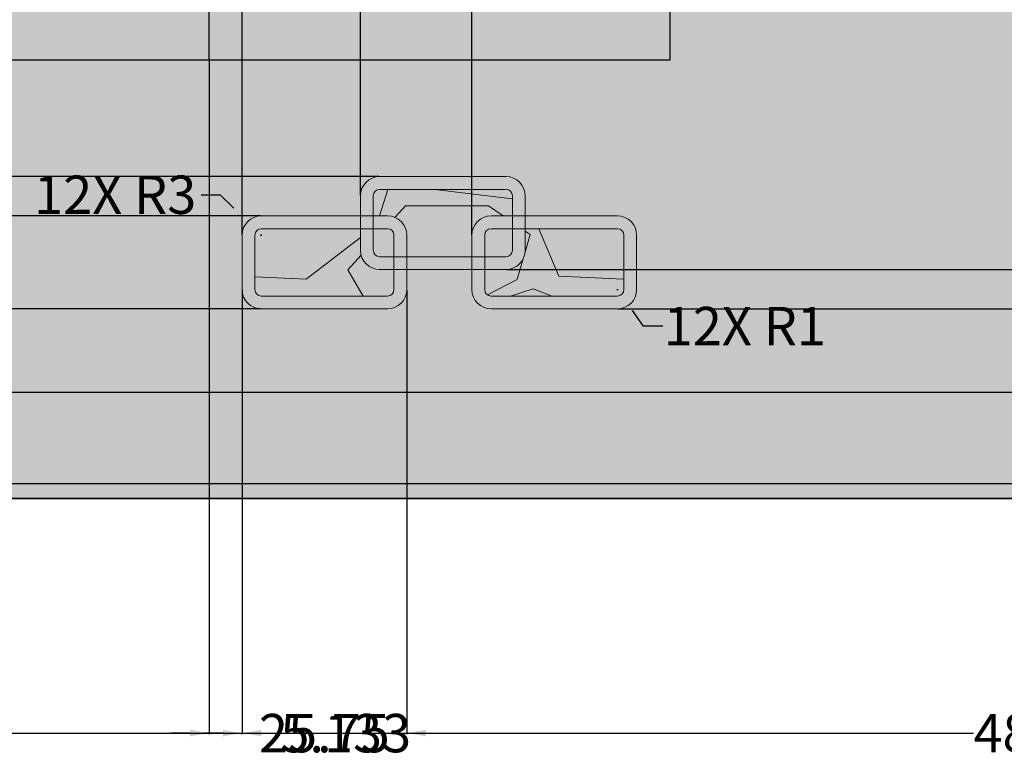
# Model space of a CAD drawing. Units: inches. Extents: x 126 to 726, y 86 to 888.
# Tile 2 of 13: x 270 to 424, y 86 to 202. Entities that reach past the tile are written whole.
import ezdxf

# ---------------------------------------------------------------- set-up
doc = ezdxf.new("R2010")
doc.units = ezdxf.units.IN
doc.header["$MEASUREMENT"] = 0
for name, color, linetype, lineweight in [('A-ANNO-DIMS', 2, 'Continuous', 18), ('A-ELEV', 7, 'Continuous', 35), ('A-ELEV-DECO', 7, 'Continuous', 18), ('A-ELEV-PATT', 8, 'Continuous', 13), ('A-GLAZ', 4, 'Continuous', 25)]:
    doc.layers.add(name, color=color, linetype=linetype, lineweight=lineweight)
doc.styles.get("Standard").update_dxf_attribs({"font": 'arial.ttf'})
doc.dimstyles.get("Standard").update_dxf_attribs({"dimtxt": 6, "dimasz": 3, "dimexe": 0.18, "dimexo": 0.0625, "dimgap": 0.09, "dimtad": 0, "dimtih": 1, "dimtoh": 1, "dimdec": 0, "dimzin": 0, "dimdsep": 46, "dimlunit": 3, "dimtxsty": 'Standard', "dimcen": 0.09, "dimadec": 0, "dimazin": 0, "dimtfac": 1, "dimtdec": 0, "dimtofl": 0, "dimtmove": 0, "dimatfit": 3, "dimfxl": 1, "dimtolj": 1, "dimtzin": 0, "dimarcsym": 0})

# ---------------------------------------------------------------- blocks, each defined once
blk = doc.blocks.new('WIN-FRAME')
for points in [[(72, 0), (0, 0), (0, 108), (72, 108)], [(63, 9), (9, 9), (9, 99), (63, 99)]]:
    blk.add_lwpolyline(points, close=True)
blk = doc.blocks.new('*D13')
at = {"layer": 'A-ANNO-DIMS', "color": 0, "lineweight": -2, "transparency": 16777216}
for p, q in [((665.97, 642.98), (665.97, 90.21)), ((185.97, 126.98), (185.97, 90.21)), ((188.97, 90.39), (419.15, 90.39)), ((662.97, 90.39), (432.8, 90.39))]:
    blk.add_line(p, q, dxfattribs=at)
at = {"layer": 'A-ANNO-DIMS', "color": 0, "transparency": 16777216}
for points in [[(188.97, 90.89), (188.97, 89.89), (185.97, 90.39)], [(662.97, 90.89), (662.97, 89.89), (665.97, 90.39)]]:
    blk.add_solid(points, dxfattribs=at)
at = {"layer": 'Defpoints', "color": 0, "transparency": 16777216}
for p in [(665.97, 643.04), (185.97, 127.04), (665.97, 90.39)]:
    blk.add_point(p, dxfattribs=at)
at = {"layer": 'A-ANNO-DIMS', "color": 0, "transparency": 16777216, "insert": (425.97, 90.39), "char_height": 6, "attachment_point": 5}
blk.add_mtext('\\A1;480', dxfattribs=at)
blk = doc.blocks.new('*D15')
at = {"layer": 'A-ANNO-DIMS', "color": 0, "lineweight": -2, "transparency": 16777216}
for p, q in [((299.6, 195.59), (149.14, 195.59)), ((149.32, 192.59), (149.32, 164.47)), ((149.32, 130.04), (149.32, 158.16)), ((185.91, 127.04), (149.14, 127.04))]:
    blk.add_line(p, q, dxfattribs=at)
at = {"layer": 'A-ANNO-DIMS', "color": 0, "transparency": 16777216}
for points in [[(148.82, 192.59), (149.82, 192.59), (149.32, 195.59)], [(148.82, 130.04), (149.82, 130.04), (149.32, 127.04)]]:
    blk.add_solid(points, dxfattribs=at)
at = {"layer": 'Defpoints', "color": 0, "transparency": 16777216}
for p in [(149.32, 195.59), (299.67, 195.59), (185.97, 127.04)]:
    blk.add_point(p, dxfattribs=at)
at = {"layer": 'A-ANNO-DIMS', "color": 0, "transparency": 16777216, "insert": (149.32, 161.31), "char_height": 6, "attachment_point": 5}
blk.add_mtext('\\A1;68.55', dxfattribs=at)
blk = doc.blocks.new('*D16')
at = {"layer": 'A-ANNO-DIMS', "color": 0, "lineweight": -2, "transparency": 16777216}
for p, q in [((299.6, 425.68), (149.14, 425.68)), ((149.32, 422.68), (149.32, 313.79)), ((149.32, 198.59), (149.32, 307.48)), ((299.6, 195.59), (149.14, 195.59))]:
    blk.add_line(p, q, dxfattribs=at)
at = {"layer": 'A-ANNO-DIMS', "color": 0, "transparency": 16777216}
for points in [[(148.82, 422.68), (149.82, 422.68), (149.32, 425.68)], [(148.82, 198.59), (149.82, 198.59), (149.32, 195.59)]]:
    blk.add_solid(points, dxfattribs=at)
at = {"layer": 'Defpoints', "color": 0, "transparency": 16777216}
for p in [(149.32, 425.68), (299.67, 425.68), (299.67, 195.59)]:
    blk.add_point(p, dxfattribs=at)
at = {"layer": 'A-ANNO-DIMS', "color": 0, "transparency": 16777216, "insert": (149.32, 310.64), "char_height": 6, "attachment_point": 5}
blk.add_mtext('\\A1;230.1', dxfattribs=at)
blk = doc.blocks.new('*D18')
at = {"layer": 'A-ANNO-DIMS', "color": 0, "lineweight": -2, "transparency": 16777216}
for p, q in [((431.28, 395.58), (149.14, 395.58)), ((149.32, 392.58), (149.32, 264.47)), ((149.32, 130.04), (149.32, 258.16)), ((185.91, 127.04), (149.14, 127.04))]:
    blk.add_line(p, q, dxfattribs=at)
at = {"layer": 'A-ANNO-DIMS', "color": 0, "transparency": 16777216}
for points in [[(148.82, 392.58), (149.82, 392.58), (149.32, 395.58)], [(148.82, 130.04), (149.82, 130.04), (149.32, 127.04)]]:
    blk.add_solid(points, dxfattribs=at)
at = {"layer": 'Defpoints', "color": 0, "transparency": 16777216}
for p in [(149.32, 395.58), (431.34, 395.58), (185.97, 127.04)]:
    blk.add_point(p, dxfattribs=at)
at = {"layer": 'A-ANNO-DIMS', "color": 0, "transparency": 16777216, "insert": (149.32, 261.31), "char_height": 6, "attachment_point": 5}
blk.add_mtext('\\A1;268.54', dxfattribs=at)
blk = doc.blocks.new('*D30')
at = {"layer": 'A-ANNO-DIMS', "color": 0, "lineweight": -2, "transparency": 16777216}
for p, q in [((299.6, 195.59), (149.14, 195.59)), ((149.32, 192.59), (149.32, 189.64)), ((149.32, 180.39), (149.32, 183.33)), ((326.24, 177.39), (149.14, 177.39))]:
    blk.add_line(p, q, dxfattribs=at)
at = {"layer": 'A-ANNO-DIMS', "color": 0, "transparency": 16777216}
for points in [[(148.82, 192.59), (149.82, 192.59), (149.32, 195.59)], [(148.82, 180.39), (149.82, 180.39), (149.32, 177.39)]]:
    blk.add_solid(points, dxfattribs=at)
at = {"layer": 'Defpoints', "color": 0, "transparency": 16777216}
for p in [(149.32, 195.59), (299.67, 195.59), (326.3, 177.39)]:
    blk.add_point(p, dxfattribs=at)
at = {"layer": 'A-ANNO-DIMS', "color": 0, "transparency": 16777216, "insert": (149.32, 186.49), "char_height": 6, "attachment_point": 5}
blk.add_mtext('\\A1;18.2', dxfattribs=at)
blk = doc.blocks.new('*D31')
at = {"layer": 'A-ANNO-DIMS', "color": 0, "lineweight": -2, "transparency": 16777216}
for p, q in [((299.67, 195.52), (299.67, 90.21)), ((304.8, 159.65), (304.8, 90.21)), ((296.67, 90.39), (293.67, 90.39)), ((307.8, 90.39), (310.8, 90.39))]:
    blk.add_line(p, q, dxfattribs=at)
at = {"layer": 'A-ANNO-DIMS', "color": 0, "transparency": 16777216}
for points in [[(296.67, 90.89), (296.67, 89.89), (299.67, 90.39)], [(307.8, 90.89), (307.8, 89.89), (304.8, 90.39)]]:
    blk.add_solid(points, dxfattribs=at)
at = {"layer": 'Defpoints', "color": 0, "transparency": 16777216}
for p in [(299.67, 195.59), (304.8, 159.71), (304.8, 90.39)]:
    blk.add_point(p, dxfattribs=at)
at = {"layer": 'A-ANNO-DIMS', "color": 0, "transparency": 16777216, "insert": (321.01, 90.39), "char_height": 6, "attachment_point": 5}
blk.add_mtext('\\A1;5.133', dxfattribs=at)
blk = doc.blocks.new('*D36')
at = {"layer": 'A-ANNO-DIMS', "color": 0, "lineweight": -2, "transparency": 16777216}
for p, q in [((304.8, 159.65), (304.8, 90.21)), ((330.55, 159.65), (330.55, 90.21)), ((301.8, 90.39), (298.8, 90.39)), ((333.55, 90.39), (336.55, 90.39))]:
    blk.add_line(p, q, dxfattribs=at)
at = {"layer": 'A-ANNO-DIMS', "color": 0, "transparency": 16777216}
for points in [[(301.8, 90.89), (301.8, 89.89), (304.8, 90.39)], [(333.55, 90.89), (333.55, 89.89), (330.55, 90.39)]]:
    blk.add_solid(points, dxfattribs=at)
at = {"layer": 'Defpoints', "color": 0, "transparency": 16777216}
for p in [(304.8, 159.71), (330.55, 159.71), (330.55, 90.39)]:
    blk.add_point(p, dxfattribs=at)
at = {"layer": 'A-ANNO-DIMS', "color": 0, "transparency": 16777216, "insert": (317.67, 90.39), "char_height": 6, "attachment_point": 5}
blk.add_mtext('\\A1;25.75', dxfattribs=at)
blk = doc.blocks.new('*D37')
at = {"layer": 'A-ANNO-DIMS', "color": 0, "lineweight": -2, "transparency": 16777216}
for p, q in [((307.74, 171.24), (149.14, 171.24)), ((149.32, 168.24), (149.32, 167.13)), ((149.32, 159.71), (149.32, 160.82)), ((307.74, 156.71), (149.14, 156.71))]:
    blk.add_line(p, q, dxfattribs=at)
at = {"layer": 'A-ANNO-DIMS', "color": 0, "transparency": 16777216}
for points in [[(148.82, 168.24), (149.82, 168.24), (149.32, 171.24)], [(148.82, 159.71), (149.82, 159.71), (149.32, 156.71)]]:
    blk.add_solid(points, dxfattribs=at)
at = {"layer": 'Defpoints', "color": 0, "transparency": 16777216}
for p in [(149.32, 171.24), (307.8, 171.24), (307.8, 156.71)]:
    blk.add_point(p, dxfattribs=at)
at = {"layer": 'A-ANNO-DIMS', "color": 0, "transparency": 16777216, "insert": (149.32, 163.98), "char_height": 6, "attachment_point": 5}
blk.add_mtext('\\A1;14.524', dxfattribs=at)
blk = doc.blocks.new('*D38')
at = {"layer": 'A-ANNO-DIMS', "color": 0, "lineweight": -2, "transparency": 16777216}
for p, q in [((304.8, 168.3), (304.8, 883.87)), ((307.8, 883.69), (320.3, 883.69)), ((323.3, 174.45), (323.3, 883.87)), ((323.3, 883.69), (326.3, 883.69))]:
    blk.add_line(p, q, dxfattribs=at)
at = {"layer": 'A-ANNO-DIMS', "color": 0, "transparency": 16777216}
for points in [[(307.8, 884.19), (307.8, 883.19), (304.8, 883.69)], [(320.3, 884.19), (320.3, 883.19), (323.3, 883.69)]]:
    blk.add_solid(points, dxfattribs=at)
at = {"layer": 'Defpoints', "color": 0, "transparency": 16777216}
for p in [(323.3, 883.69), (323.3, 174.39), (304.8, 168.24)]:
    blk.add_point(p, dxfattribs=at)
at = {"layer": 'A-ANNO-DIMS', "color": 0, "transparency": 16777216, "insert": (338.59, 883.69), "char_height": 6, "attachment_point": 5}
blk.add_mtext('\\A1;18.505', dxfattribs=at)
blk = doc.blocks.new('*D39')
at = {"layer": 'A-ANNO-DIMS', "color": 0, "lineweight": -2, "transparency": 16777216}
for p, q in [((323.3, 174.45), (323.3, 883.87)), ((326.3, 883.69), (337.74, 883.69)), ((340.74, 168.3), (340.74, 883.87)), ((340.74, 883.69), (343.74, 883.69))]:
    blk.add_line(p, q, dxfattribs=at)
at = {"layer": 'A-ANNO-DIMS', "color": 0, "transparency": 16777216}
for points in [[(326.3, 884.19), (326.3, 883.19), (323.3, 883.69)], [(337.74, 884.19), (337.74, 883.19), (340.74, 883.69)]]:
    blk.add_solid(points, dxfattribs=at)
at = {"layer": 'Defpoints', "color": 0, "transparency": 16777216}
for p in [(340.74, 883.69), (323.3, 174.39), (340.74, 168.24)]:
    blk.add_point(p, dxfattribs=at)
at = {"layer": 'A-ANNO-DIMS', "color": 0, "transparency": 16777216, "insert": (355.99, 883.69), "char_height": 6, "attachment_point": 5}
blk.add_mtext('\\A1;17.434', dxfattribs=at)
blk = doc.blocks.new('*D40')
at = {"layer": 'A-ANNO-DIMS', "color": 0, "lineweight": -2, "transparency": 16777216}
for p, q in [((702.62, 165.86), (702.62, 168.86)), ((702.62, 168.86), (705.62, 168.86)), ((346.12, 162.86), (702.8, 162.86)), ((363.55, 156.71), (702.8, 156.71)), ((702.62, 153.71), (702.62, 150.71))]:
    blk.add_line(p, q, dxfattribs=at)
at = {"layer": 'A-ANNO-DIMS', "color": 0, "transparency": 16777216}
for points in [[(702.12, 165.86), (703.12, 165.86), (702.62, 162.86)], [(702.12, 153.71), (703.12, 153.71), (702.62, 156.71)]]:
    blk.add_solid(points, dxfattribs=at)
at = {"layer": 'Defpoints', "color": 0, "transparency": 16777216}
for p in [(346.06, 162.86), (702.62, 162.86), (363.49, 156.71)]:
    blk.add_point(p, dxfattribs=at)
at = {"layer": 'A-ANNO-DIMS', "color": 0, "transparency": 16777216, "insert": (715.86, 168.86), "char_height": 6, "attachment_point": 5}
blk.add_mtext('\\A1;6.149', dxfattribs=at)
blk = doc.blocks.new('*D79')
at = {"layer": 'A-ANNO-DIMS', "color": 0, "lineweight": -2, "transparency": 16777216}
for p, q in [((149.32, 132.35), (149.32, 135.35)), ((437.91, 129.35), (149.14, 129.35)), ((485.91, 127.04), (149.14, 127.04)), ((149.32, 124.04), (149.32, 121.04)), ((149.32, 121.04), (146.32, 121.04))]:
    blk.add_line(p, q, dxfattribs=at)
at = {"layer": 'A-ANNO-DIMS', "color": 0, "transparency": 16777216}
for points in [[(148.82, 132.35), (149.82, 132.35), (149.32, 129.35)], [(148.82, 124.04), (149.82, 124.04), (149.32, 127.04)]]:
    blk.add_solid(points, dxfattribs=at)
at = {"layer": 'Defpoints', "color": 0, "transparency": 16777216}
for p in [(437.97, 129.35), (149.32, 127.04), (485.97, 127.04)]:
    blk.add_point(p, dxfattribs=at)
at = {"layer": 'A-ANNO-DIMS', "color": 0, "transparency": 16777216, "insert": (136.64, 121.04), "char_height": 6, "attachment_point": 5}
blk.add_mtext('\\A1;2.311', dxfattribs=at)
blk = doc.blocks.new('*D80')
at = {"layer": 'A-ANNO-DIMS', "color": 0, "lineweight": -2, "transparency": 16777216}
for p, q in [((437.91, 143.66), (149.14, 143.66)), ((149.32, 140.66), (149.32, 139.66)), ((149.32, 132.35), (149.32, 133.35)), ((437.91, 129.35), (149.14, 129.35))]:
    blk.add_line(p, q, dxfattribs=at)
at = {"layer": 'A-ANNO-DIMS', "color": 0, "transparency": 16777216}
for points in [[(148.82, 140.66), (149.82, 140.66), (149.32, 143.66)], [(148.82, 132.35), (149.82, 132.35), (149.32, 129.35)]]:
    blk.add_solid(points, dxfattribs=at)
at = {"layer": 'Defpoints', "color": 0, "transparency": 16777216}
for p in [(149.32, 143.66), (437.97, 143.66), (437.97, 129.35)]:
    blk.add_point(p, dxfattribs=at)
at = {"layer": 'A-ANNO-DIMS', "color": 0, "transparency": 16777216, "insert": (149.32, 136.51), "char_height": 6, "attachment_point": 5}
blk.add_mtext('\\A1;14.31', dxfattribs=at)
blk = doc.blocks.new('*D83')
at = {"layer": 'A-ANNO-DIMS', "color": 0, "lineweight": -2, "transparency": 16777216}
for p, q in [((298.38, 174.55), (301.38, 174.55)), ((301.38, 174.55), (303.52, 172.44)), ((307.71, 168.24), (307.89, 168.24)), ((307.8, 168.15), (307.8, 168.33))]:
    blk.add_line(p, q, dxfattribs=at)
at = {"layer": 'A-ANNO-DIMS', "color": 0, "transparency": 16777216}
blk.add_solid([(303.87, 172.8), (303.17, 172.09), (305.66, 170.34)], dxfattribs=at)
at = {"layer": 'Defpoints', "color": 0, "transparency": 16777216}
for p in [(305.66, 170.34), (307.8, 168.24)]:
    blk.add_point(p, dxfattribs=at)
at = {"layer": 'A-ANNO-DIMS', "color": 0, "transparency": 16777216, "insert": (284.96, 174.55), "char_height": 6, "attachment_point": 5}
blk.add_mtext('\\A1;12X R3', dxfattribs=at)
blk = doc.blocks.new('*D84')
at = {"layer": 'A-ANNO-DIMS', "color": 0, "lineweight": -2, "transparency": 16777216}
for p, q in [((363.4, 159.71), (363.58, 159.71)), ((363.49, 159.62), (363.49, 159.8)), ((367.57, 154.02), (365.82, 156.46)), ((370.57, 154.02), (367.57, 154.02))]:
    blk.add_line(p, q, dxfattribs=at)
at = {"layer": 'A-ANNO-DIMS', "color": 0, "transparency": 16777216}
blk.add_solid([(366.22, 156.75), (365.41, 156.17), (364.07, 158.9)], dxfattribs=at)
at = {"layer": 'Defpoints', "color": 0, "transparency": 16777216}
for p in [(363.49, 159.71), (364.07, 158.9)]:
    blk.add_point(p, dxfattribs=at)
at = {"layer": 'A-ANNO-DIMS', "color": 0, "transparency": 16777216, "insert": (383.41, 154.02), "char_height": 6, "attachment_point": 5}
blk.add_mtext('\\A1;12X R1', dxfattribs=at)

msp = doc.modelspace()

# ---------------------------------------------------------------- hatches: boundary and pattern name
at = {"layer": 'A-ELEV-PATT'}
h = msp.add_hatch(color=256, dxfattribs=at)
h.dxf.hatch_style = 1
h.paths.add_polyline_path([(437.9749, 499.1312), (485.9749, 499.1312), (485.9749, 501.4423), (437.9749, 501.4423), (437.9749, 513.4423), (485.9749, 513.4423), (485.9749, 515.7534), (437.9749, 515.7534), (437.9749, 527.7534), (485.9749, 527.7534), (485.9749, 530.0646), (437.9749, 530.0646), (437.9749, 542.0646), (485.9749, 542.0646), (485.9749, 544.3757), (437.9749, 544.3757), (437.9749, 556.3757), (485.9749, 556.3757), (485.9749, 558.6868), (437.9749, 558.6868), (437.9749, 570.6868), (485.9749, 570.6868), (485.9749, 572.9979), (437.9749, 572.9979), (437.9749, 584.9979), (485.9749, 584.9979), (485.9749, 587.309), (437.9749, 587.309), (437.9749, 595.0424), (429.9749, 595.0424), (429.9749, 607.0424), (437.9749, 607.0424), (437.9749, 615.9312), (437.9749, 630.2423), (437.9749, 642.2423), (485.9749, 642.2423), (485.9749, 644.5534), (437.9749, 644.5534), (437.9749, 656.5534), (485.9749, 656.5534), (485.9749, 658.8645), (437.9749, 658.8645), (437.9749, 670.8645), (485.9749, 670.8645), (485.9749, 673.1757), (437.9749, 673.1757), (437.9749, 685.1757), (485.9749, 685.1757), (485.9749, 687.4868), (437.9749, 687.4868), (437.9749, 699.4868), (485.9749, 699.4868), (485.9749, 701.7979), (437.9749, 701.7979), (437.9749, 713.7979), (485.9749, 713.7979), (485.9749, 716.109), (437.9749, 716.109), (437.9749, 728.109), (485.9749, 728.109), (485.9749, 730.4201), (437.9749, 730.4201), (437.9749, 742.4201), (485.9749, 742.4201), (485.9749, 744.7312), (437.9749, 744.7312), (437.9749, 756.7312), (485.9749, 756.7312), (485.9749, 759.0423), (437.9749, 759.0423), (437.9749, 771.0423), (485.9749, 771.0423), (485.9749, 773.3534), (437.9749, 773.3534), (437.9749, 785.3534), (485.9749, 785.3534), (485.9749, 787.6645), (437.9749, 787.6645), (437.9749, 799.6645), (485.9749, 799.6645), (485.9749, 801.9756), (437.9749, 801.9756), (437.9749, 811.2868), (485.9749, 811.2868), (485.9749, 813.9756), (437.9749, 813.9756), (437.9749, 825.9756), (485.9749, 825.9756), (485.9749, 835.0424), (233.9749, 835.0424), (233.9749, 606.5846), (185.9749, 606.5846), (185.9749, 597.5846), (233.9749, 597.5846), (233.9749, 585.5846), (185.9749, 585.5846), (185.9749, 580.5846), (233.9749, 580.5846), (233.9749, 568.5846), (185.9749, 568.5846), (185.9749, 563.5846), (431.3386, 563.5846), (431.3386, 545.5846), (233.9749, 545.5846), (233.9749, 413.5846), (431.3386, 413.5846), (431.3386, 395.5846), (185.9749, 395.5846), (185.9749, 386.5846), (233.9749, 386.5846), (233.9749, 374.5846), (185.9749, 374.5846), (185.9749, 369.5846), (233.9749, 369.5846), (233.9749, 357.5846), (185.9749, 357.5846), (185.9749, 352.5846), (233.9749, 352.5846), (233.9749, 340.5846), (185.9749, 340.5846), (185.9749, 331.5846), (233.9749, 331.5846), (233.9749, 127.0424), (485.9749, 127.0424), (485.9749, 129.3535), (437.9749, 129.3535), (437.9749, 141.3535), (485.9749, 141.3535), (485.9749, 143.6646), (437.9749, 143.6646), (437.9749, 155.6646), (485.9749, 155.6646), (485.9749, 157.9757), (437.9749, 157.9757), (437.9749, 169.9757), (485.9749, 169.9757), (485.9749, 172.2868), (437.9749, 172.2868), (437.9749, 184.2868), (485.9749, 184.2868), (485.9749, 186.5979), (437.9749, 186.5979), (437.9749, 198.5979), (485.9749, 198.5979), (485.9749, 200.909), (437.9749, 200.909), (437.9749, 212.909), (485.9749, 212.909), (485.9749, 215.2201), (437.9749, 215.2201), (437.9749, 227.2201), (485.9749, 227.2201), (485.9749, 229.5312), (437.9749, 229.5312), (437.9749, 241.5312), (485.9749, 241.5312), (485.9749, 243.8424), (437.9749, 243.8424), (437.9749, 255.8424), (485.9749, 255.8424), (485.9749, 258.1535), (437.9749, 258.1535), (437.9749, 270.1535), (485.9749, 270.1535), (485.9749, 272.4646), (437.9749, 272.4646), (437.9749, 284.4646), (485.9749, 284.4646), (485.9749, 286.7757), (437.9749, 286.7757), (437.9749, 298.7757), (485.9749, 298.7757), (485.9749, 301.0868), (437.9749, 301.0868), (437.9749, 313.0868), (485.9749, 313.0868), (485.9749, 315.3979), (437.9749, 315.3979), (437.9749, 327.3979), (485.9749, 327.3979), (485.9749, 329.709), (437.9749, 329.709), (437.9749, 341.709), (485.9749, 341.709), (485.9749, 344.0201), (437.9749, 344.0201), (437.9749, 355.0424), (429.9749, 355.0424), (429.9749, 367.0424), (437.9749, 367.0424), (437.9749, 372.6423), (437.9749, 386.9535), (437.9749, 401.2646), (437.9749, 413.2646), (485.9749, 413.2646), (485.9749, 415.5757), (437.9749, 415.5757), (437.9749, 427.5757), (485.9749, 427.5757), (485.9749, 429.8868), (437.9749, 429.8868), (437.9749, 441.8868), (485.9749, 441.8868), (485.9749, 444.1979), (437.9749, 444.1979), (437.9749, 456.1979), (485.9749, 456.1979), (485.9749, 458.509), (437.9749, 458.509), (437.9749, 470.509), (485.9749, 470.509), (485.9749, 472.8201), (437.9749, 472.8201), (437.9749, 484.8201), (485.9749, 484.8201), (485.9749, 487.1312), (437.9749, 487.1312)])
h.paths.add_polyline_path([(299.6658, 533.6845), (371.6658, 533.6845), (371.6658, 425.6845), (299.6658, 425.6845)], flags=16)
h.paths.add_polyline_path([(308.6658, 524.6845), (362.6658, 524.6845), (362.6658, 434.6845), (308.6658, 434.6845)], flags=0)
h.paths.add_polyline_path([(317.7956, 603.3211, -0.4129833), (306.8418, 614.321, -0.94403766), (328.769, 615.5845, -0.04423165), (330.7031, 615.4048, -0.89973713), (352.5798, 615.6161, -0.4129833), (363.5336, 604.6162, -0.94403766), (341.6064, 603.3528, -0.04423165), (339.6723, 603.5324, -0.89973713)], flags=16)
h.paths.add_polyline_path([(319.7228, 604.5846, -0.02633223), (319.7726, 605.5306, -0.47905713), (308.8418, 614.321, -1), (326.8418, 614.321, -0.02633223), (326.7919, 613.375, -0.17413188), (332.826, 612.5948, -0.04918553), (332.6526, 614.3527, -1), (350.6526, 614.3527, -0.02633223), (350.6028, 613.4067, -0.47905713), (361.5336, 604.6162, -1), (343.5336, 604.6162, -0.02633223), (343.5834, 605.5622, -0.17413188), (337.5494, 606.3424, -0.04918553), (337.7228, 604.5846, -1)], flags=0)
h.paths.add_polyline_path([(328.769, 355.6561, -0.04423165), (330.7031, 355.4765, -0.89973713), (352.5798, 355.6878, -0.4129833), (363.5336, 344.6879, -0.94403766), (341.6064, 343.4244, -0.04423165), (339.6723, 343.604, -0.89973713), (317.7956, 343.3927, -0.4129833), (306.8418, 354.3926, -0.94403766)], flags=16)
h.paths.add_polyline_path([(326.8418, 354.3926, -0.02633223), (326.7919, 353.4466, -0.17413188), (332.826, 352.6664, -0.04918553), (332.6526, 354.4243, -1), (350.6526, 354.4243, -0.02633223), (350.6028, 353.4783, -0.47905713), (361.5336, 344.6879, -1), (343.5336, 344.6879, -0.02633223), (343.5834, 345.6339, -0.17413188), (337.5494, 346.4141, -0.04918553), (337.7228, 344.6562, -1), (319.7228, 344.6562, -0.02633223), (319.7726, 345.6022, -0.47905713), (308.8418, 354.3926, -1)], flags=0)
h.paths.add_polyline_path([(299.3189, 655.3527), (299.3189, 763.3527), (371.3189, 763.3527), (371.3189, 655.3527)], flags=16)
h.paths.add_polyline_path([(308.3189, 664.3527), (308.3189, 754.3527), (362.3189, 754.3527), (362.3189, 664.3527)], flags=0)
h.paths.add_polyline_path([(299.6658, 303.5875), (371.6658, 303.5875), (371.6658, 195.5875), (299.6658, 195.5875)], flags=16)
h.paths.add_polyline_path([(308.6658, 294.5875), (362.6658, 294.5875), (362.6658, 204.5875), (308.6658, 204.5875)], flags=0)
h.paths.add_polyline_path([(326.3038, 177.3867), (346.055, 177.3867, -0.41421356), (349.055, 174.3867), (349.055, 171.2378), (363.489, 171.2378, -0.41421356), (366.489, 168.2378), (366.489, 159.7133, -0.41421356), (363.489, 156.7133), (343.7379, 156.7133, -0.41421356), (340.7379, 159.7133), (340.7379, 162.8622), (330.5504, 162.8622), (330.5504, 159.7133, -0.41421356), (327.5504, 156.7133), (307.7992, 156.7133, -0.41421356), (304.7992, 159.7133), (304.7992, 168.2378, -0.41421356), (307.7992, 171.2378), (323.3038, 171.2378), (323.3038, 174.3867, -0.41421356)], flags=16)
h.paths.add_polyline_path([(326.3038, 175.3867), (346.055, 175.3867, -0.41421356), (347.055, 174.3867), (347.055, 169.2378), (363.489, 169.2378, -0.41421356), (364.489, 168.2378), (364.489, 159.7133, -0.41421356), (363.489, 158.7133), (343.7379, 158.7133, -0.41421356), (342.7379, 159.7133), (342.7379, 164.8622), (328.5504, 164.8622), (328.5504, 159.7133, -0.41421356), (327.5504, 158.7133), (307.7992, 158.7133, -0.41421356), (306.7992, 159.7133), (306.7992, 168.2378, -0.41421356), (307.7992, 169.2378), (325.3038, 169.2378), (325.3038, 174.3867, -0.41421356)], flags=0)
h = msp.add_hatch(dxfattribs=at)
h.set_pattern_fill('GRAVEL', color=256, scale=40)
h.paths.add_polyline_path([(437.9749, 642.2423), (485.9749, 642.2423), (485.9749, 644.5534), (437.9749, 644.5534), (437.9749, 656.5534), (485.9749, 656.5534), (485.9749, 658.8645), (437.9749, 658.8645), (437.9749, 670.8645), (485.9749, 670.8645), (485.9749, 673.1757), (437.9749, 673.1757), (437.9749, 685.1757), (485.9749, 685.1757), (485.9749, 687.4868), (437.9749, 687.4868), (437.9749, 699.4868), (485.9749, 699.4868), (485.9749, 701.7979), (437.9749, 701.7979), (437.9749, 713.7979), (485.9749, 713.7979), (485.9749, 716.109), (437.9749, 716.109), (437.9749, 728.109), (485.9749, 728.109), (485.9749, 730.4201), (437.9749, 730.4201), (437.9749, 742.4201), (485.9749, 742.4201), (485.9749, 744.7312), (437.9749, 744.7312), (437.9749, 756.7312), (485.9749, 756.7312), (485.9749, 759.0423), (437.9749, 759.0423), (437.9749, 771.0423), (485.9749, 771.0423), (485.9749, 773.3534), (437.9749, 773.3534), (437.9749, 785.3534), (485.9749, 785.3534), (485.9749, 787.6645), (437.9749, 787.6645), (437.9749, 799.6645), (485.9749, 799.6645), (485.9749, 801.9756), (437.9749, 801.9756), (437.9749, 811.2868), (485.9749, 811.2868), (485.9749, 813.9756), (437.9749, 813.9756), (437.9749, 825.9756), (485.9749, 825.9756), (485.9749, 835.0424), (233.9749, 835.0424), (233.9749, 606.5846), (185.9749, 606.5846), (185.9749, 597.5846), (233.9749, 597.5846), (233.9749, 585.5846), (185.9749, 585.5846), (185.9749, 580.5846), (233.9749, 580.5846), (233.9749, 568.5846), (185.9749, 568.5846), (185.9749, 563.5846), (431.3386, 563.5846), (431.3386, 545.5846), (233.9749, 545.5846), (233.9749, 413.5846), (431.3386, 413.5846), (431.3386, 395.5846), (185.9749, 395.5846), (185.9749, 386.5846), (233.9749, 386.5846), (233.9749, 374.5846), (185.9749, 374.5846), (185.9749, 369.5846), (233.9749, 369.5846), (233.9749, 357.5846), (185.9749, 357.5846), (185.9749, 352.5846), (233.9749, 352.5846), (233.9749, 340.5846), (185.9749, 340.5846), (185.9749, 331.5846), (233.9749, 331.5846), (233.9749, 127.0424), (485.9749, 127.0424), (485.9749, 129.3535), (437.9749, 129.3535), (437.9749, 141.3535), (485.9749, 141.3535), (485.9749, 143.6646), (437.9749, 143.6646), (437.9749, 155.6646), (485.9749, 155.6646), (485.9749, 157.9757), (437.9749, 157.9757), (437.9749, 169.9757), (485.9749, 169.9757), (485.9749, 172.2868), (437.9749, 172.2868), (437.9749, 184.2868), (485.9749, 184.2868), (485.9749, 186.5979), (437.9749, 186.5979), (437.9749, 198.5979), (485.9749, 198.5979), (485.9749, 200.909), (437.9749, 200.909), (437.9749, 212.909), (485.9749, 212.909), (485.9749, 215.2201), (437.9749, 215.2201), (437.9749, 227.2201), (485.9749, 227.2201), (485.9749, 229.5312), (437.9749, 229.5312), (437.9749, 241.5312), (485.9749, 241.5312), (485.9749, 243.8424), (437.9749, 243.8424), (437.9749, 255.8424), (485.9749, 255.8424), (485.9749, 258.1535), (437.9749, 258.1535), (437.9749, 270.1535), (485.9749, 270.1535), (485.9749, 272.4646), (437.9749, 272.4646), (437.9749, 284.4646), (485.9749, 284.4646), (485.9749, 286.7757), (437.9749, 286.7757), (437.9749, 298.7757), (485.9749, 298.7757), (485.9749, 301.0868), (437.9749, 301.0868), (437.9749, 313.0868), (485.9749, 313.0868), (485.9749, 315.3979), (437.9749, 315.3979), (437.9749, 327.3979), (485.9749, 327.3979), (485.9749, 329.709), (437.9749, 329.709), (437.9749, 341.709), (485.9749, 341.709), (485.9749, 344.0201), (437.9749, 344.0201), (437.9749, 355.0424), (429.9749, 355.0424), (429.9749, 367.0424), (437.9749, 367.0424), (437.9749, 372.6423), (437.9749, 386.9535), (437.9749, 401.2646), (437.9749, 413.2646), (485.9749, 413.2646), (485.9749, 415.5757), (437.9749, 415.5757), (437.9749, 427.5757), (485.9749, 427.5757), (485.9749, 429.8868), (437.9749, 429.8868), (437.9749, 441.8868), (485.9749, 441.8868), (485.9749, 444.1979), (437.9749, 444.1979), (437.9749, 456.1979), (485.9749, 456.1979), (485.9749, 458.509), (437.9749, 458.509), (437.9749, 470.509), (485.9749, 470.509), (485.9749, 472.8201), (437.9749, 472.8201), (437.9749, 484.8201), (485.9749, 484.8201), (485.9749, 487.1312), (437.9749, 487.1312), (437.9749, 499.1312), (485.9749, 499.1312), (485.9749, 501.4423), (437.9749, 501.4423), (437.9749, 513.4423), (485.9749, 513.4423), (485.9749, 515.7534), (437.9749, 515.7534), (437.9749, 527.7534), (485.9749, 527.7534), (485.9749, 530.0646), (437.9749, 530.0646), (437.9749, 542.0646), (485.9749, 542.0646), (485.9749, 544.3757), (437.9749, 544.3757), (437.9749, 556.3757), (485.9749, 556.3757), (485.9749, 558.6868), (437.9749, 558.6868), (437.9749, 570.6868), (485.9749, 570.6868), (485.9749, 572.9979), (437.9749, 572.9979), (437.9749, 584.9979), (485.9749, 584.9979), (485.9749, 587.309), (437.9749, 587.309), (437.9749, 595.0424), (429.9749, 595.0424), (429.9749, 607.0424), (437.9749, 607.0424), (437.9749, 615.9312), (437.9749, 630.2423)])
h.paths.add_polyline_path([(371.3189, 655.3527), (299.3189, 655.3527), (299.3189, 763.3527), (371.3189, 763.3527)], flags=16)
h.paths.add_polyline_path([(363.5336, 604.6162, -0.94403766), (341.6064, 603.3528, -0.04423165), (339.6723, 603.5324, -0.89973713), (317.7956, 603.3211, -0.4129833), (306.8418, 614.321, -0.94403766), (328.769, 615.5845, -0.04423165), (330.7031, 615.4048, -0.89973713), (352.5798, 615.6161, -0.4129833)], flags=16)
h.paths.add_polyline_path([(361.5336, 604.6162, -1), (343.5336, 604.6162, -0.02633223), (343.5834, 605.5622, -0.17413188), (337.5494, 606.3424, -0.04918553), (337.7228, 604.5846, -1), (319.7228, 604.5846, -0.02633223), (319.7726, 605.5306, -0.47905713), (308.8418, 614.321, -1), (326.8418, 614.321, -0.02633223), (326.7919, 613.375, -0.17413188), (332.826, 612.5948, -0.04918553), (332.6526, 614.3527, -1), (350.6526, 614.3527, -0.02633223), (350.6028, 613.4067, -0.47905713)], flags=0)
h.paths.add_polyline_path([(362.3189, 664.3527), (308.3189, 664.3527), (308.3189, 754.3527), (362.3189, 754.3527)], flags=0)
h.paths.add_polyline_path([(371.6658, 533.6845), (371.6658, 425.6845), (299.6658, 425.6845), (299.6658, 533.6845)], flags=16)
h.paths.add_polyline_path([(362.6658, 524.6845), (362.6658, 434.6845), (308.6658, 434.6845), (308.6658, 524.6845)], flags=0)
h.paths.add_polyline_path([(352.5798, 355.6878, -0.4129833), (363.5336, 344.6879, -0.94403766), (341.6064, 343.4244, -0.04423165), (339.6723, 343.604, -0.89973713), (317.7956, 343.3927, -0.4129833), (306.8418, 354.3926, -0.94403766), (328.769, 355.6561, -0.04423165), (330.7031, 355.4765, -0.89973713)], flags=16)
h.paths.add_polyline_path([(350.6526, 354.4243, -0.02633223), (350.6028, 353.4783, -0.47905713), (361.5336, 344.6879, -1), (343.5336, 344.6879, -0.02633223), (343.5834, 345.6339, -0.17413188), (337.5494, 346.4141, -0.04918553), (337.7228, 344.6562, -1), (319.7228, 344.6562, -0.02633223), (319.7726, 345.6022, -0.47905713), (308.8418, 354.3926, -1), (326.8418, 354.3926, -0.02633223), (326.7919, 353.4466, -0.17413188), (332.826, 352.6664, -0.04918553), (332.6526, 354.4243, -1)], flags=0)
h.paths.add_polyline_path([(371.6658, 303.5875), (371.6658, 195.5875), (299.6658, 195.5875), (299.6658, 303.5875)], flags=16)
h.paths.add_polyline_path([(362.6658, 294.5875), (362.6658, 204.5875), (308.6658, 204.5875), (308.6658, 294.5875)], flags=0)
h.paths.add_polyline_path([(346.055, 177.3867, -0.41421356), (349.055, 174.3867), (349.055, 171.2378), (363.489, 171.2378, -0.41421356), (366.489, 168.2378), (366.489, 159.7133, -0.41421356), (363.489, 156.7133), (343.7379, 156.7133, -0.41421356), (340.7379, 159.7133), (340.7379, 162.8622), (330.5504, 162.8622), (330.5504, 159.7133, -0.41421356), (327.5504, 156.7133), (307.7992, 156.7133, -0.41421356), (304.7992, 159.7133), (304.7992, 168.2378, -0.41421356), (307.7992, 171.2378), (323.3038, 171.2378), (323.3038, 174.3867, -0.41421356), (326.3038, 177.3867)], flags=16)
h.paths.add_polyline_path([(346.055, 175.3867, -0.41421356), (347.055, 174.3867), (347.055, 169.2378), (363.489, 169.2378, -0.41421356), (364.489, 168.2378), (364.489, 159.7133, -0.41421356), (363.489, 158.7133), (343.7379, 158.7133, -0.41421356), (342.7379, 159.7133), (342.7379, 164.8622), (328.5504, 164.8622), (328.5504, 159.7133, -0.41421356), (327.5504, 158.7133), (307.7992, 158.7133, -0.41421356), (306.7992, 159.7133), (306.7992, 168.2378, -0.41421356), (307.7992, 169.2378), (325.3038, 169.2378), (325.3038, 174.3867, -0.41421356), (326.3038, 175.3867)], flags=0)
h = msp.add_hatch(color=256, dxfattribs=at)
h.dxf.hatch_style = 1
h.paths.add_polyline_path([(343.7379, 171.2378), (347.055, 171.2378), (347.055, 174.3867, 0.41421356), (346.055, 175.3867), (326.3038, 175.3867, 0.41421356), (325.3038, 174.3867), (325.3038, 171.2378), (327.5504, 171.2378, -0.41421356), (330.5504, 168.2378), (330.5504, 164.8622), (340.7379, 164.8622), (340.7379, 168.2378, -0.41421356)])
h.paths.add_polyline_path([(328.5504, 162.8622), (326.3038, 162.8622, -0.41421356), (323.3038, 165.8622), (323.3038, 169.2378), (307.7992, 169.2378, 0.41421356), (306.7992, 168.2378), (306.7992, 159.7133, 0.41421356), (307.7992, 158.7133), (327.5504, 158.7133, 0.41421356), (328.5504, 159.7133)])
h.paths.add_polyline_path([(328.5504, 168.2378, 0.41421356), (327.5504, 169.2378), (325.3038, 169.2378), (325.3038, 165.8622, 0.41421356), (326.3038, 164.8622), (328.5504, 164.8622)], flags=17)
h.paths.add_polyline_path([(364.489, 168.2378, 0.41421356), (363.489, 169.2378), (349.055, 169.2378), (349.055, 165.8622, -0.41421356), (346.055, 162.8622), (342.7379, 162.8622), (342.7379, 159.7133, 0.41421356), (343.7379, 158.7133), (363.489, 158.7133, 0.41421356), (364.489, 159.7133)])
h.paths.add_polyline_path([(347.055, 169.2378), (343.7379, 169.2378, 0.41421356), (342.7379, 168.2378), (342.7379, 164.8622), (346.055, 164.8622, 0.41421356), (347.055, 165.8622)], flags=17)
h.paths.add_polyline_path([(361.5336, 344.6879, 0.4111475), (352.6279, 353.6874, -0.34414474), (343.5998, 343.598, 0.94107412)])
h.paths.add_polyline_path([(332.6665, 354.9249, -0.28599337), (339.6784, 345.6435, 0.05271891), (341.5583, 345.4248, -0.34414474), (350.5864, 355.5141, 0.91517696)])
h.paths.add_polyline_path([(308.8418, 354.3926, 0.4111475), (317.7475, 345.3931, -0.34414474), (326.7756, 355.4825, 0.94107412)])
h.paths.add_polyline_path([(326.7919, 353.4466, 0.32288595), (319.7726, 345.6022, 0.32288595)])
h.paths.add_polyline_path([(330.697, 353.437, 0.05271891), (328.8171, 353.6557, -0.34414474), (319.789, 343.5663, 0.91517696), (337.7088, 344.1556, -0.28599337)])
h.paths.add_polyline_path([(332.826, 352.6664, 0.22909031), (337.5494, 346.4141, 0.22909031)], flags=17)
h.paths.add_polyline_path([(350.6028, 353.4783, 0.32288595), (343.5834, 345.6339, 0.32288595)])
h.paths.add_polyline_path([(332.6665, 614.8533, -0.28599337), (339.6784, 605.5719, 0.05271891), (341.5583, 605.3532, -0.34414474), (350.5864, 615.4425, 0.91517696)])
h.paths.add_polyline_path([(308.8418, 614.321, 0.4111475), (317.7475, 605.3215, -0.34414474), (326.7756, 615.4109, 0.94107412)])
h.paths.add_polyline_path([(337.7088, 604.084, -0.28599337), (330.697, 613.3654, 0.05271891), (328.8171, 613.5841, -0.34414474), (319.789, 603.4947, 0.91517696)])
h.paths.add_polyline_path([(361.5336, 604.6162, 0.4111475), (352.6279, 613.6157, -0.34414474), (343.5998, 603.5264, 0.94107412)])
h.paths.add_polyline_path([(350.6028, 613.4067, 0.32288595), (343.5834, 605.5622, 0.32288595)])
h.paths.add_polyline_path([(332.826, 612.5948, 0.22909031), (337.5494, 606.3424, 0.22909031)], flags=17)
h.paths.add_polyline_path([(326.7919, 613.375, 0.32288595), (319.7726, 605.5306, 0.32288595)])
h = msp.add_hatch(color=256, dxfattribs=at)
h.dxf.hatch_style = 1
h.paths.add_polyline_path([(371.6658, 303.5875), (299.6658, 303.5875), (299.6658, 195.5875), (371.6658, 195.5875)])
h.paths.add_polyline_path([(362.6658, 294.5875), (362.6658, 204.5875), (308.6658, 204.5875), (308.6658, 294.5875)], flags=16)
h.paths.add_polyline_path([(366.489, 159.7133), (366.489, 168.2378, 0.41421356), (363.489, 171.2378), (349.055, 171.2378), (349.055, 169.2378), (363.489, 169.2378, -0.41421356), (364.489, 168.2378), (364.489, 159.7133, -0.41421356), (363.489, 158.7133), (343.7379, 158.7133, -0.41421356), (342.7379, 159.7133), (342.7379, 162.8622), (340.7379, 162.8622), (340.7379, 159.7133, 0.41421356), (343.7379, 156.7133), (363.489, 156.7133, 0.41421356)])
h.paths.add_polyline_path([(349.055, 171.2378), (347.055, 171.2378), (347.055, 169.2378), (349.055, 169.2378)], flags=17)
h.paths.add_polyline_path([(349.055, 169.2378), (347.055, 169.2378), (347.055, 165.8622, -0.41421356), (346.055, 164.8622), (342.7379, 164.8622), (342.7379, 162.8622), (346.055, 162.8622, 0.41421356), (349.055, 165.8622)], flags=17)
h.paths.add_polyline_path([(342.7379, 164.8622), (340.7379, 164.8622), (340.7379, 162.8622), (342.7379, 162.8622)], flags=17)
h.paths.add_polyline_path([(342.7379, 168.2378, -0.41421356), (343.7379, 169.2378), (347.055, 169.2378), (347.055, 171.2378), (343.7379, 171.2378, 0.41421356), (340.7379, 168.2378), (340.7379, 164.8622), (342.7379, 164.8622)], flags=17)
h.paths.add_polyline_path([(349.055, 174.3867, 0.41421356), (346.055, 177.3867), (326.3038, 177.3867, 0.41421356), (323.3038, 174.3867), (323.3038, 171.2378), (325.3038, 171.2378), (325.3038, 174.3867, -0.41421356), (326.3038, 175.3867), (346.055, 175.3867, -0.41421356), (347.055, 174.3867), (347.055, 171.2378), (349.055, 171.2378)])
h.paths.add_polyline_path([(327.5504, 171.2378), (325.3038, 171.2378), (325.3038, 169.2378), (327.5504, 169.2378, -0.41421356), (328.5504, 168.2378), (328.5504, 164.8622), (330.5504, 164.8622), (330.5504, 168.2378, 0.41421356)], flags=17)
h.paths.add_polyline_path([(325.3038, 171.2378), (323.3038, 171.2378), (323.3038, 169.2378), (325.3038, 169.2378)], flags=17)
h.paths.add_polyline_path([(325.3038, 169.2378), (323.3038, 169.2378), (323.3038, 165.8622, 0.41421356), (326.3038, 162.8622), (328.5504, 162.8622), (328.5504, 164.8622), (326.3038, 164.8622, -0.41421356), (325.3038, 165.8622)], flags=17)
h.paths.add_polyline_path([(330.5504, 164.8622), (328.5504, 164.8622), (328.5504, 162.8622), (330.5504, 162.8622)], flags=17)
h.paths.add_polyline_path([(340.7379, 164.8622), (330.5504, 164.8622), (330.5504, 162.8622), (340.7379, 162.8622)])
h.paths.add_polyline_path([(330.5504, 162.8622), (328.5504, 162.8622), (328.5504, 159.7133, -0.41421356), (327.5504, 158.7133), (307.7992, 158.7133, -0.41421356), (306.7992, 159.7133), (306.7992, 168.2378, -0.41421356), (307.7992, 169.2378), (323.3038, 169.2378), (323.3038, 171.2378), (307.7992, 171.2378, 0.41421356), (304.7992, 168.2378), (304.7992, 159.7133, 0.41421356), (307.7992, 156.7133), (327.5504, 156.7133, 0.41421356), (330.5504, 159.7133)])
h = msp.add_hatch(dxfattribs=at)
h.set_pattern_fill('GRAVEL', color=256, scale=50)
h.paths.add_polyline_path([(343.7379, 171.2378), (347.055, 171.2378), (347.055, 174.3867, 0.41421356), (346.055, 175.3867), (326.3038, 175.3867, 0.41421356), (325.3038, 174.3867), (325.3038, 171.2378), (327.5504, 171.2378, -0.41421356), (330.5504, 168.2378), (330.5504, 164.8622), (340.7379, 164.8622), (340.7379, 168.2378, -0.41421356)])
h.paths.add_polyline_path([(323.3038, 165.8622), (323.3038, 169.2378), (307.7992, 169.2378, 0.41421356), (306.7992, 168.2378), (306.7992, 159.7133, 0.41421356), (307.7992, 158.7133), (327.5504, 158.7133, 0.41421356), (328.5504, 159.7133), (328.5504, 162.8622), (326.3038, 162.8622, -0.41421356)])
h.paths.add_polyline_path([(364.489, 168.2378, 0.41421356), (363.489, 169.2378), (349.055, 169.2378), (349.055, 165.8622, -0.41421356), (346.055, 162.8622), (342.7379, 162.8622), (342.7379, 159.7133, 0.41421356), (343.7379, 158.7133), (363.489, 158.7133, 0.41421356), (364.489, 159.7133)])

# ---------------------------------------------------------------- linework, layer by layer
at = {"layer": 'A-ELEV'}
msp.add_line((185.9749, 127.0424), (660.0469, 127.0424), dxfattribs=at)
at = {"layer": 'A-ELEV-DECO'}
for points in [[(323.3038, 174.3867, -0.41421356), (326.3038, 177.3867), (346.055, 177.3867, -0.41421356), (349.055, 174.3867), (349.055, 165.8622, -0.41421356), (346.055, 162.8622), (326.3038, 162.8622, -0.41421356), (323.3038, 165.8622)], [(325.3038, 174.3867, -0.41421356), (326.3038, 175.3867), (346.055, 175.3867, -0.41421356), (347.055, 174.3867), (347.055, 165.8622, -0.41421356), (346.055, 164.8622), (326.3038, 164.8622, -0.41421356), (325.3038, 165.8622)], [(304.7992, 168.2378, -0.41421356), (307.7992, 171.2378), (327.5504, 171.2378, -0.41421356), (330.5504, 168.2378), (330.5504, 159.7133, -0.41421356), (327.5504, 156.7133), (307.7992, 156.7133, -0.41421356), (304.7992, 159.7133)], [(340.7379, 168.2378, -0.41421356), (343.7379, 171.2378), (363.489, 171.2378, -0.41421356), (366.489, 168.2378), (366.489, 159.7133, -0.41421356), (363.489, 156.7133), (343.7379, 156.7133, -0.41421356), (340.7379, 159.7133)], [(306.7992, 168.2378, -0.41421356), (307.7992, 169.2378), (327.5504, 169.2378, -0.41421356), (328.5504, 168.2378), (328.5504, 159.7133, -0.41421356), (327.5504, 158.7133), (307.7992, 158.7133, -0.41421356), (306.7992, 159.7133)], [(342.7379, 168.2378, -0.41421356), (343.7379, 169.2378), (363.489, 169.2378, -0.41421356), (364.489, 168.2378), (364.489, 159.7133, -0.41421356), (363.489, 158.7133), (343.7379, 158.7133, -0.41421356), (342.7379, 159.7133)]]:
    msp.add_lwpolyline(points, format="xyb", close=True, dxfattribs=at)

# ---------------------------------------------------------------- block references
at = {"layer": 'A-GLAZ'}
msp.add_blockref('WIN-FRAME', (299.6659, 195.5878), dxfattribs=at)

# ---------------------------------------------------------------- dimensions: what is measured, and where the dimension line sits
at = {"layer": 'A-ANNO-DIMS'}
for base, p1, p2, override, picture, middle in [((323.3038, 883.6924), (304.7992, 168.2378), (323.3038, 174.3867), {"dimdec": 3, "dimlfac": 1, "dimrnd": 0, "dimzin": 0, "dimdsep": 46, "dimlunit": 2}, '*D38', (338.5882, 883.6924)), ((340.7379, 883.6924), (323.3038, 174.3867), (340.7379, 168.2378), {"dimdec": 3, "dimlfac": 1, "dimrnd": 0, "dimzin": 0, "dimdsep": 46, "dimlunit": 2}, '*D39', (355.9875, 883.6924)), ((665.9749, 90.3924), (185.9749, 127.0424), (665.9749, 643.0424), {"dimdec": 0, "dimlfac": 1, "dimrnd": 0, "dimzin": 0, "dimdsep": 46, "dimlunit": 2}, '*D13', (425.9749, 90.3924)), ((304.7992, 90.3924), (299.6658, 195.5875), (304.7992, 159.7133), {"dimdec": 3, "dimlfac": 1, "dimrnd": 0, "dimzin": 0, "dimdsep": 46, "dimlunit": 2}, '*D31', (321.0127, 90.3924)), ((330.5504, 90.3924), (304.7992, 159.7133), (330.5504, 159.7133), {"dimdec": 2, "dimlfac": 1, "dimrnd": 0, "dimzin": 0, "dimdsep": 46, "dimlunit": 2}, '*D36', (317.6748, 90.3924))]:
    dim = msp.add_linear_dim(base=base, p1=p1, p2=p2, dimstyle='Standard', override=override, dxfattribs=at)
    dim.commit()
    dim.dimension.update_dxf_attribs({"geometry": picture, "text_midpoint": middle})
for base, p1, p2, override, picture, middle in [((149.3249, 425.6845), (299.6658, 195.5875), (299.6658, 425.6845), {"dimdec": 1, "dimlfac": 1, "dimrnd": 0, "dimzin": 0, "dimdsep": 46, "dimlunit": 2}, '*D16', (149.3249, 310.636)), ((149.3249, 395.5846), (185.9749, 127.0424), (431.3386, 395.5846), {"dimdec": 2, "dimlfac": 1, "dimrnd": 0, "dimzin": 0, "dimdsep": 46, "dimlunit": 2}, '*D18', (149.3249, 261.3135)), ((149.3249, 195.5875), (185.9749, 127.0424), (299.6658, 195.5875), {"dimdec": 2, "dimlfac": 1, "dimrnd": 0, "dimzin": 0, "dimdsep": 46, "dimlunit": 2}, '*D15', (149.3249, 161.3149)), ((149.3249, 195.5875), (326.3038, 177.3867), (299.6658, 195.5875), {"dimdec": 1, "dimlfac": 1, "dimrnd": 0, "dimzin": 0, "dimdsep": 46, "dimlunit": 2}, '*D30', (149.3249, 186.4871)), ((702.6249, 162.8622), (363.489, 156.7133), (346.055, 162.8622), {"dimdec": 3, "dimlfac": 1, "dimrnd": 0, "dimzin": 0, "dimdsep": 46, "dimlunit": 2}, '*D40', (715.8609, 168.8622)), ((149.32491, 171.23781), (307.79919, 156.71334), (307.79919, 171.23781), {"dimdec": 3, "dimlfac": 1, "dimrnd": 0, "dimzin": 0, "dimdsep": 46, "dimlunit": 2}, '*D37', (149.32491, 163.97557)), ((149.3249, 143.6646), (437.9749, 129.3535), (437.9749, 143.6646), {"dimdec": 2, "dimlfac": 1, "dimrnd": 0, "dimzin": 0, "dimdsep": 46, "dimlunit": 2}, '*D80', (149.3249, 136.509)), ((149.3249, 127.0424), (437.9749, 129.3535), (485.9749, 127.0424), {"dimdec": 3, "dimlfac": 1, "dimrnd": 0, "dimzin": 0, "dimdsep": 46, "dimlunit": 2}, '*D79', (136.6394, 121.0424))]:
    dim = msp.add_linear_dim(base=base, p1=p1, p2=p2, angle=90, dimstyle='Standard', override=override, dxfattribs=at)
    dim.commit()
    dim.dimension.update_dxf_attribs({"geometry": picture, "text_midpoint": middle})
for center, mpoint, picture, middle in [((307.7992, 168.2378), (305.6593, 170.3404), '*D83', (284.9572, 174.5455)), ((363.489, 159.7133), (364.0714, 158.9004), '*D84', (383.4084, 154.0227))]:
    dim = msp.add_radius_dim(center=center, mpoint=mpoint, text='12X <>', dimstyle='Standard', override={"dimdec": 0, "dimlfac": 1, "dimrnd": 0, "dimzin": 0, "dimdsep": 46, "dimlunit": 2}, dxfattribs=at)
    dim.commit()
    dim.dimension.update_dxf_attribs({"geometry": picture, "text_midpoint": middle})

doc.saveas('drawing.dxf')
